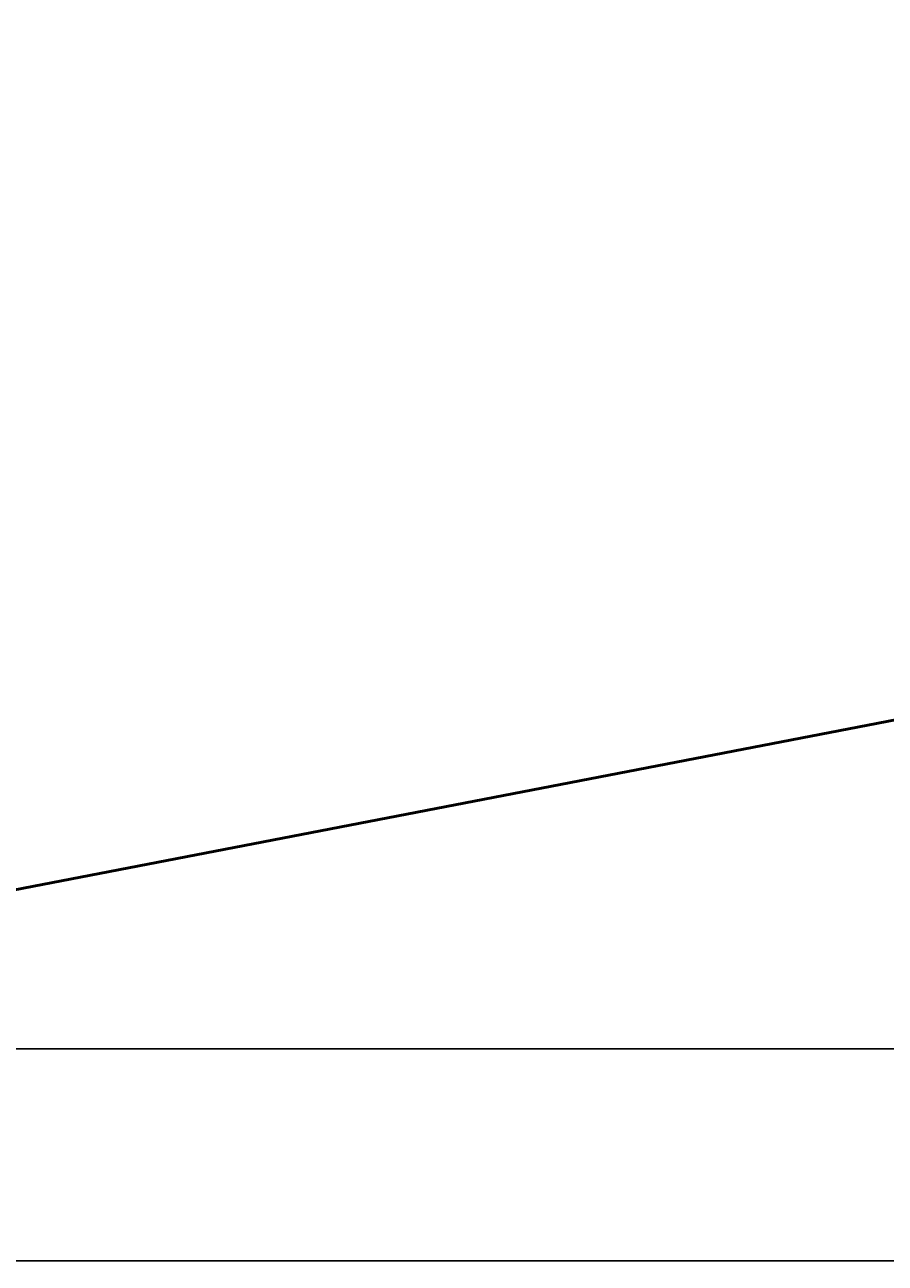
# Model space of a CAD drawing. Units: inches. Extents: x 457 to 775, y 319 to 541.
# Tile 8 of 12: x 623 to 694, y 319 to 421. Entities that reach past the tile are written whole.
import ezdxf

# ---------------------------------------------------------------- set-up
doc = ezdxf.new("R2010")
doc.units = ezdxf.units.IN
doc.header["$MEASUREMENT"] = 0
doc.layers.add('M-DIMS', color=2, linetype='Continuous', lineweight=18)
doc.layers.add('M-OUTL', color=7, linetype='Continuous', lineweight=50)
doc.styles.get("Standard").update_dxf_attribs({"font": 'arial.ttf'})
doc.dimstyles.get("Standard").update_dxf_attribs({"dimtxt": 0.18, "dimasz": 0.18, "dimexe": 0.18, "dimexo": 0.0625, "dimgap": 0.09, "dimtad": 0, "dimtih": 1, "dimtoh": 1, "dimdec": 4, "dimzin": 0, "dimdsep": 46, "dimtxsty": 'Standard', "dimcen": 0.09, "dimadec": 0, "dimazin": 0, "dimtfac": 1, "dimtdec": 4, "dimtofl": 0, "dimtmove": 0, "dimatfit": 3, "dimfxl": 1, "dimtolj": 1, "dimtzin": 0, "dimarcsym": 0})

# ---------------------------------------------------------------- blocks, each defined once
blk = doc.blocks.new('*D2')
at = {"layer": 'Defpoints', "color": 0, "transparency": 16777216}
for p in [(756.93, 375.7), (474.31, 336.7), (756.93, 319.3)]:
    blk.add_point(p, dxfattribs=at)
at = {"layer": 'M-DIMS', "color": 0, "lineweight": -2, "transparency": 16777216}
for p, q in [((756.93, 375.63), (756.93, 319.12)), ((474.31, 336.63), (474.31, 319.12)), ((474.49, 319.3), (615.22, 319.3)), ((756.75, 319.3), (616.01, 319.3))]:
    blk.add_line(p, q, dxfattribs=at)
at = {"layer": 'M-DIMS', "color": 0, "transparency": 16777216}
for points in [[(474.49, 319.33), (474.49, 319.27), (474.31, 319.3)], [(756.75, 319.33), (756.75, 319.27), (756.93, 319.3)]]:
    blk.add_solid(points, dxfattribs=at)
at = {"layer": 'M-DIMS', "color": 0, "transparency": 16777216, "insert": (615.62, 319.3), "char_height": 0.18, "attachment_point": 5}
blk.add_mtext('\\A1;282.6', dxfattribs=at)
blk = doc.blocks.new('*D3')
at = {"layer": 'Defpoints', "color": 0, "transparency": 16777216}
for p in [(456.91, 523.21), (646, 523.21), (474.31, 336.7)]:
    blk.add_point(p, dxfattribs=at)
at = {"layer": 'M-DIMS', "color": 0, "lineweight": -2, "transparency": 16777216}
for p, q in [((645.94, 523.21), (456.73, 523.21)), ((456.91, 523.03), (456.91, 430.14)), ((456.91, 336.88), (456.91, 429.77)), ((474.24, 336.7), (456.73, 336.7))]:
    blk.add_line(p, q, dxfattribs=at)
at = {"layer": 'M-DIMS', "color": 0, "transparency": 16777216}
for points in [[(456.88, 523.03), (456.94, 523.03), (456.91, 523.21)], [(456.88, 336.88), (456.94, 336.88), (456.91, 336.7)]]:
    blk.add_solid(points, dxfattribs=at)
at = {"layer": 'M-DIMS', "color": 0, "transparency": 16777216, "insert": (456.91, 429.95), "char_height": 0.18, "attachment_point": 5}
blk.add_mtext('\\A1;186.5', dxfattribs=at)
blk = doc.blocks.new('*D9')
at = {"layer": 'Defpoints', "color": 0, "transparency": 16777216}
for p in [(756.93, 375.7), (774.33, 375.7), (554.93, 336.7)]:
    blk.add_point(p, dxfattribs=at)
at = {"layer": 'M-DIMS', "color": 0, "lineweight": -2, "transparency": 16777216}
for p, q in [((756.99, 375.7), (774.51, 375.7)), ((774.33, 375.52), (774.33, 356.38)), ((774.33, 336.88), (774.33, 356.01)), ((554.99, 336.7), (774.51, 336.7))]:
    blk.add_line(p, q, dxfattribs=at)
at = {"layer": 'M-DIMS', "color": 0, "transparency": 16777216}
for points in [[(774.3, 375.52), (774.36, 375.52), (774.33, 375.7)], [(774.3, 336.88), (774.36, 336.88), (774.33, 336.7)]]:
    blk.add_solid(points, dxfattribs=at)
at = {"layer": 'M-DIMS', "color": 0, "transparency": 16777216, "insert": (774.33, 356.2), "char_height": 0.18, "attachment_point": 5}
blk.add_mtext('\\A1;39', dxfattribs=at)

msp = doc.modelspace()

# ---------------------------------------------------------------- linework, layer by layer
at = {"layer": 'M-OUTL'}
msp.add_line((554.931, 336.696), (756.931, 375.696), dxfattribs=at)

# ---------------------------------------------------------------- dimensions: what is measured, and where the dimension line sits
at = {"layer": 'M-DIMS'}
for base, p1, p2, override, picture, middle in [((456.906, 523.213), (474.306, 336.696), (646.001, 523.213), {"dimdec": 1, "dimlfac": 1, "dimrnd": 0, "dimzin": 0, "dimdsep": 46, "dimlunit": 2}, '*D3', (456.906, 429.954)), ((774.331, 375.696), (554.931, 336.696), (756.931, 375.696), {"dimdec": 0, "dimlfac": 1, "dimrnd": 0, "dimzin": 0, "dimdsep": 46, "dimlunit": 2}, '*D9', (774.331, 356.196))]:
    dim = msp.add_linear_dim(base=base, p1=p1, p2=p2, angle=90, dimstyle='Standard', override=override, dxfattribs=at)
    dim.commit()
    dim.dimension.update_dxf_attribs({"geometry": picture, "text_midpoint": middle})
dim = msp.add_linear_dim(base=(756.931, 319.296), p1=(474.306, 336.696), p2=(756.931, 375.696), dimstyle='Standard', override={"dimdec": 1, "dimlfac": 1, "dimrnd": 0, "dimzin": 0, "dimdsep": 46, "dimlunit": 2}, dxfattribs=at)
dim.commit()
dim.dimension.update_dxf_attribs({"geometry": '*D2', "text_midpoint": (615.619, 319.296)})

doc.saveas('drawing.dxf')
